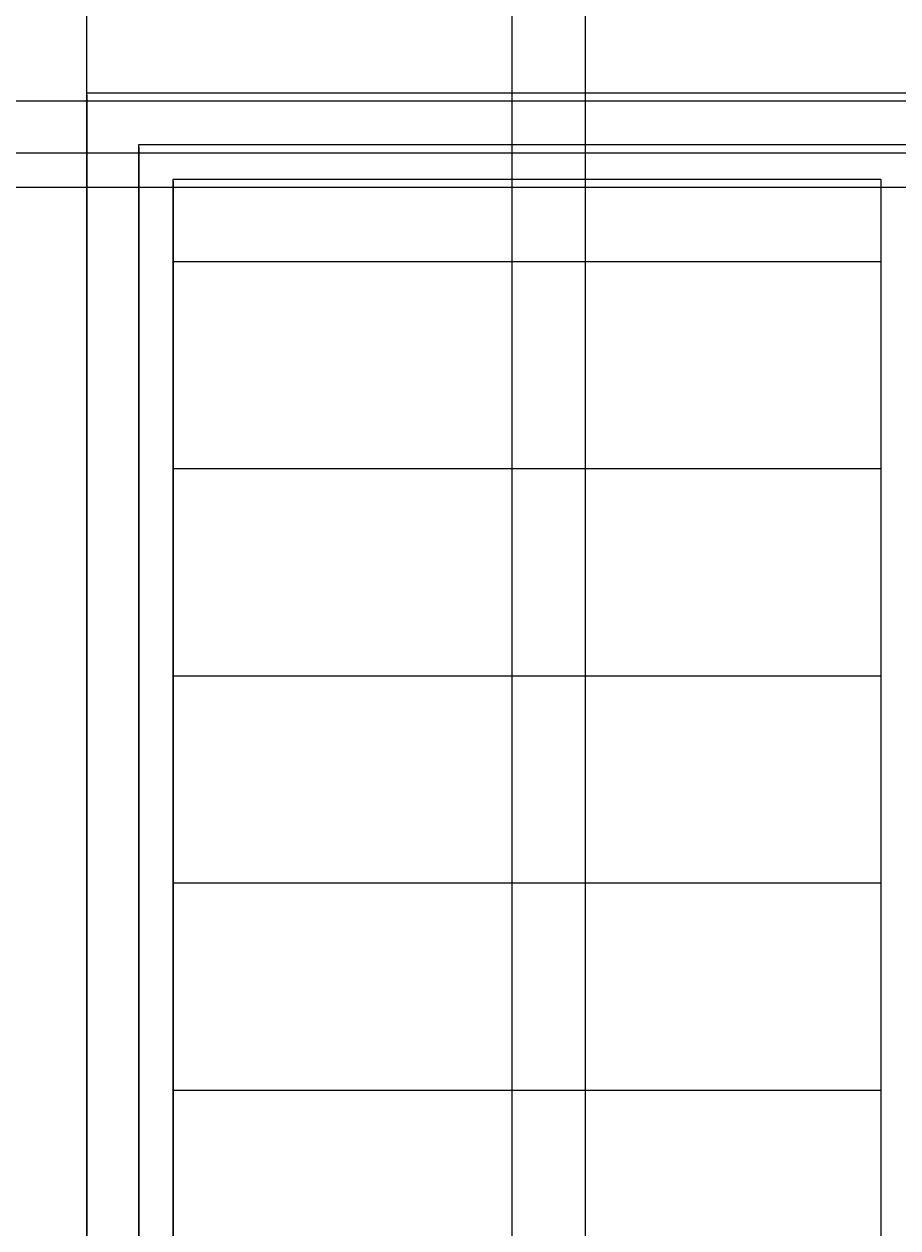
# Model space of a CAD drawing. Units: inches. Extents: x -6 to 289, y -8 to 323.
# Tile 70 of 107: x 186 to 212, y 194 to 229. Entities that reach past the tile are written whole.
import ezdxf

# ---------------------------------------------------------------- set-up
doc = ezdxf.new("R2010")
doc.units = ezdxf.units.IN
doc.header["$MEASUREMENT"] = 0
for name, color, linetype, lineweight in [('A-ANNO-DIMS', 2, 'Continuous', 18), ('A-ELEV-PATT', 8, 'Continuous', 13), ('A-GLAZ', 4, 'Continuous', 25)]:
    doc.layers.add(name, color=color, linetype=linetype, lineweight=lineweight)
doc.styles.get("Standard").update_dxf_attribs({"font": 'arial.ttf'})
doc.dimstyles.get("Standard").update_dxf_attribs({"dimtxt": 0.18, "dimasz": 0.18, "dimexe": 0.18, "dimexo": 0.0625, "dimgap": 0.09, "dimtad": 0, "dimtih": 1, "dimtoh": 1, "dimdec": 4, "dimzin": 0, "dimdsep": 46, "dimtxsty": 'Standard', "dimcen": 0.09, "dimadec": 0, "dimazin": 0, "dimtfac": 1, "dimtdec": 4, "dimtofl": 0, "dimtmove": 0, "dimatfit": 3, "dimfxl": 1, "dimtolj": 1, "dimtzin": 0, "dimarcsym": 0})

# ---------------------------------------------------------------- blocks, each defined once
blk = doc.blocks.new('*D12')
at = {"layer": 'A-ANNO-DIMS', "color": 0, "lineweight": -2, "transparency": 16777216}
for p, q in [((168.883, 226.717), (168.883, 322.969)), ((188.292, 226.951), (188.292, 322.969)), ((169.063, 322.789), (178.22, 322.789)), ((188.112, 322.789), (178.955, 322.789))]:
    blk.add_line(p, q, dxfattribs=at)
at = {"layer": 'A-ANNO-DIMS', "color": 0, "transparency": 16777216}
for points in [[(169.063, 322.819), (169.063, 322.759), (168.883, 322.789)], [(188.112, 322.819), (188.112, 322.759), (188.292, 322.789)]]:
    blk.add_solid(points, dxfattribs=at)
at = {"layer": 'Defpoints', "color": 0, "transparency": 16777216}
for p in [(188.292, 322.789), (168.883, 226.654), (188.292, 226.889)]:
    blk.add_point(p, dxfattribs=at)
at = {"layer": 'A-ANNO-DIMS', "color": 0, "transparency": 16777216, "insert": (178.588, 322.789), "char_height": 0.18, "attachment_point": 5}
blk.add_mtext('\\A1;19.41', dxfattribs=at)
blk = doc.blocks.new('*D13')
at = {"layer": 'A-ANNO-DIMS', "color": 0, "lineweight": -2, "transparency": 16777216}
for p, q in [((188.292, 226.951), (188.292, 322.969)), ((236.292, 226.951), (236.292, 322.969)), ((188.472, 322.789), (212.069, 322.789)), ((236.112, 322.789), (212.515, 322.789))]:
    blk.add_line(p, q, dxfattribs=at)
at = {"layer": 'A-ANNO-DIMS', "color": 0, "transparency": 16777216}
for points in [[(188.472, 322.819), (188.472, 322.759), (188.292, 322.789)], [(236.112, 322.819), (236.112, 322.759), (236.292, 322.789)]]:
    blk.add_solid(points, dxfattribs=at)
at = {"layer": 'Defpoints', "color": 0, "transparency": 16777216}
for p in [(236.292, 322.789), (188.292, 226.889), (236.292, 226.889)]:
    blk.add_point(p, dxfattribs=at)
at = {"layer": 'A-ANNO-DIMS', "color": 0, "transparency": 16777216, "insert": (212.292, 322.789), "char_height": 0.18, "attachment_point": 5}
blk.add_mtext('\\A1;48', dxfattribs=at)
blk = doc.blocks.new('*D25')
at = {"layer": 'A-ANNO-DIMS', "color": 0, "lineweight": -2, "transparency": 16777216}
for p, q in [((126.946, 226.654), (288.653, 226.654)), ((288.473, 226.474), (288.473, 202.836)), ((288.473, 178.834), (288.473, 202.472)), ((126.946, 178.654), (288.653, 178.654))]:
    blk.add_line(p, q, dxfattribs=at)
at = {"layer": 'A-ANNO-DIMS', "color": 0, "transparency": 16777216}
for points in [[(288.443, 226.474), (288.503, 226.474), (288.473, 226.654)], [(288.443, 178.834), (288.503, 178.834), (288.473, 178.654)]]:
    blk.add_solid(points, dxfattribs=at)
at = {"layer": 'Defpoints', "color": 0, "transparency": 16777216}
for p in [(126.883, 226.654), (288.473, 226.654), (126.883, 178.654)]:
    blk.add_point(p, dxfattribs=at)
at = {"layer": 'A-ANNO-DIMS', "color": 0, "transparency": 16777216, "insert": (288.473, 202.654), "char_height": 0.18, "attachment_point": 5}
blk.add_mtext('\\A1;48', dxfattribs=at)
blk = doc.blocks.new('*D26')
at = {"layer": 'A-ANNO-DIMS', "color": 0, "lineweight": -2, "transparency": 16777216}
for p, q in [((247.226, 247.289), (288.653, 247.289)), ((288.473, 247.109), (288.473, 237.153)), ((288.473, 226.834), (288.473, 236.789)), ((126.946, 226.654), (288.653, 226.654))]:
    blk.add_line(p, q, dxfattribs=at)
at = {"layer": 'A-ANNO-DIMS', "color": 0, "transparency": 16777216}
for points in [[(288.443, 247.109), (288.503, 247.109), (288.473, 247.289)], [(288.443, 226.834), (288.503, 226.834), (288.473, 226.654)]]:
    blk.add_solid(points, dxfattribs=at)
at = {"layer": 'Defpoints', "color": 0, "transparency": 16777216}
for p in [(247.164, 247.289), (288.473, 247.289), (126.883, 226.654)]:
    blk.add_point(p, dxfattribs=at)
at = {"layer": 'A-ANNO-DIMS', "color": 0, "transparency": 16777216, "insert": (288.473, 236.971), "char_height": 0.18, "attachment_point": 5}
blk.add_mtext('\\A1;20.635', dxfattribs=at)
blk = doc.blocks.new('*D37')
at = {"layer": 'A-ANNO-DIMS', "color": 0, "lineweight": -2, "transparency": 16777216}
for p, q in [((166.446, 224.154), (288.653, 224.154)), ((288.473, 223.974), (288.473, 202.836)), ((288.473, 181.334), (288.473, 202.472)), ((166.446, 181.154), (288.653, 181.154))]:
    blk.add_line(p, q, dxfattribs=at)
at = {"layer": 'A-ANNO-DIMS', "color": 0, "transparency": 16777216}
for points in [[(288.443, 223.974), (288.503, 223.974), (288.473, 224.154)], [(288.443, 181.334), (288.503, 181.334), (288.473, 181.154)]]:
    blk.add_solid(points, dxfattribs=at)
at = {"layer": 'Defpoints', "color": 0, "transparency": 16777216}
for p in [(166.383, 224.154), (288.473, 224.154), (166.383, 181.154)]:
    blk.add_point(p, dxfattribs=at)
at = {"layer": 'A-ANNO-DIMS', "color": 0, "transparency": 16777216, "insert": (288.473, 202.654), "char_height": 0.18, "attachment_point": 5}
blk.add_mtext('\\A1;43', dxfattribs=at)
blk = doc.blocks.new('*D38')
at = {"layer": 'A-ANNO-DIMS', "color": 0, "lineweight": -2, "transparency": 16777216}
for p, q in [((167.446, 225.154), (288.653, 225.154)), ((288.473, 224.974), (288.473, 224.834)), ((288.473, 224.334), (288.473, 224.474)), ((166.446, 224.154), (288.653, 224.154))]:
    blk.add_line(p, q, dxfattribs=at)
at = {"layer": 'A-ANNO-DIMS', "color": 0, "transparency": 16777216}
for points in [[(288.443, 224.974), (288.503, 224.974), (288.473, 225.154)], [(288.443, 224.334), (288.503, 224.334), (288.473, 224.154)]]:
    blk.add_solid(points, dxfattribs=at)
at = {"layer": 'Defpoints', "color": 0, "transparency": 16777216}
for p in [(167.383, 225.154), (288.473, 225.154), (166.383, 224.154)]:
    blk.add_point(p, dxfattribs=at)
at = {"layer": 'A-ANNO-DIMS', "color": 0, "transparency": 16777216, "insert": (288.473, 224.654), "char_height": 0.18, "attachment_point": 5}
blk.add_mtext('\\A1;1', dxfattribs=at)
blk = doc.blocks.new('*D39')
at = {"layer": 'A-ANNO-DIMS', "color": 0, "lineweight": -2, "transparency": 16777216}
for p, q in [((168.946, 226.654), (288.653, 226.654)), ((288.473, 226.474), (288.473, 226.086)), ((288.473, 225.334), (288.473, 225.722)), ((167.446, 225.154), (288.653, 225.154))]:
    blk.add_line(p, q, dxfattribs=at)
at = {"layer": 'A-ANNO-DIMS', "color": 0, "transparency": 16777216}
for points in [[(288.443, 226.474), (288.503, 226.474), (288.473, 226.654)], [(288.443, 225.334), (288.503, 225.334), (288.473, 225.154)]]:
    blk.add_solid(points, dxfattribs=at)
at = {"layer": 'Defpoints', "color": 0, "transparency": 16777216}
for p in [(168.883, 226.654), (288.473, 226.654), (167.383, 225.154)]:
    blk.add_point(p, dxfattribs=at)
at = {"layer": 'A-ANNO-DIMS', "color": 0, "transparency": 16777216, "insert": (288.473, 225.904), "char_height": 0.18, "attachment_point": 5}
blk.add_mtext('\\A1;1.5', dxfattribs=at)
blk = doc.blocks.new('*D40')
at = {"layer": 'A-ANNO-DIMS', "color": 0, "lineweight": -2, "transparency": 16777216}
for p, q in [((188.292, 226.826), (188.292, -8.391)), ((189.792, 225.326), (189.792, -8.391)), ((188.472, -8.211), (188.796, -8.211)), ((189.612, -8.211), (189.288, -8.211))]:
    blk.add_line(p, q, dxfattribs=at)
at = {"layer": 'A-ANNO-DIMS', "color": 0, "transparency": 16777216}
for points in [[(188.472, -8.181), (188.472, -8.241), (188.292, -8.211)], [(189.612, -8.181), (189.612, -8.241), (189.792, -8.211)]]:
    blk.add_solid(points, dxfattribs=at)
at = {"layer": 'Defpoints', "color": 0, "transparency": 16777216}
for p in [(188.292, 226.889), (189.792, 225.389), (189.792, -8.211)]:
    blk.add_point(p, dxfattribs=at)
at = {"layer": 'A-ANNO-DIMS', "color": 0, "transparency": 16777216, "insert": (189.042, -8.211), "char_height": 0.18, "attachment_point": 5}
blk.add_mtext('\\A1;1.5', dxfattribs=at)
blk = doc.blocks.new('*D41')
at = {"layer": 'A-ANNO-DIMS', "color": 0, "lineweight": -2, "transparency": 16777216}
for p, q in [((189.792, 225.326), (189.792, -8.391)), ((190.792, 224.326), (190.792, -8.391)), ((189.972, -8.211), (190.169, -8.211)), ((190.612, -8.211), (190.415, -8.211))]:
    blk.add_line(p, q, dxfattribs=at)
at = {"layer": 'A-ANNO-DIMS', "color": 0, "transparency": 16777216}
for points in [[(189.972, -8.181), (189.972, -8.241), (189.792, -8.211)], [(190.612, -8.181), (190.612, -8.241), (190.792, -8.211)]]:
    blk.add_solid(points, dxfattribs=at)
at = {"layer": 'Defpoints', "color": 0, "transparency": 16777216}
for p in [(189.792, 225.389), (190.792, 224.389), (190.792, -8.211)]:
    blk.add_point(p, dxfattribs=at)
at = {"layer": 'A-ANNO-DIMS', "color": 0, "transparency": 16777216, "insert": (190.292, -8.211), "char_height": 0.18, "attachment_point": 5}
blk.add_mtext('\\A1;1', dxfattribs=at)
blk = doc.blocks.new('*D42')
at = {"layer": 'A-ANNO-DIMS', "color": 0, "lineweight": -2, "transparency": 16777216}
for p, q in [((190.792, 224.326), (190.792, -8.391)), ((211.292, 224.326), (211.292, -8.391)), ((190.972, -8.211), (200.716, -8.211)), ((211.112, -8.211), (201.368, -8.211))]:
    blk.add_line(p, q, dxfattribs=at)
at = {"layer": 'A-ANNO-DIMS', "color": 0, "transparency": 16777216}
for points in [[(190.972, -8.181), (190.972, -8.241), (190.792, -8.211)], [(211.112, -8.181), (211.112, -8.241), (211.292, -8.211)]]:
    blk.add_solid(points, dxfattribs=at)
at = {"layer": 'Defpoints', "color": 0, "transparency": 16777216}
for p in [(190.792, 224.389), (211.292, 224.389), (211.292, -8.211)]:
    blk.add_point(p, dxfattribs=at)
at = {"layer": 'A-ANNO-DIMS', "color": 0, "transparency": 16777216, "insert": (201.042, -8.211), "char_height": 0.18, "attachment_point": 5}
blk.add_mtext('\\A1;20.5', dxfattribs=at)
blk = doc.blocks.new('*D43')
at = {"layer": 'A-ANNO-DIMS', "color": 0, "lineweight": -2, "transparency": 16777216}
for p, q in [((211.292, 224.326), (211.292, -8.391)), ((212.292, 224.326), (212.292, -8.391)), ((211.472, -8.211), (211.669, -8.211)), ((212.112, -8.211), (211.915, -8.211))]:
    blk.add_line(p, q, dxfattribs=at)
at = {"layer": 'A-ANNO-DIMS', "color": 0, "transparency": 16777216}
for points in [[(211.472, -8.181), (211.472, -8.241), (211.292, -8.211)], [(212.112, -8.181), (212.112, -8.241), (212.292, -8.211)]]:
    blk.add_solid(points, dxfattribs=at)
at = {"layer": 'Defpoints', "color": 0, "transparency": 16777216}
for p in [(211.292, 224.389), (212.292, 224.389), (212.292, -8.211)]:
    blk.add_point(p, dxfattribs=at)
at = {"layer": 'A-ANNO-DIMS', "color": 0, "transparency": 16777216, "insert": (211.792, -8.211), "char_height": 0.18, "attachment_point": 5}
blk.add_mtext('\\A1;1', dxfattribs=at)
blk = doc.blocks.new('*D79')
at = {"layer": 'A-ANNO-DIMS', "color": 0, "lineweight": -2, "transparency": 16777216}
for p, q in [((171.296, 118.033), (171.296, 322.969)), ((188.292, 116.842), (188.292, 322.969)), ((171.476, 322.789), (179.339, 322.789)), ((188.112, 322.789), (180.249, 322.789))]:
    blk.add_line(p, q, dxfattribs=at)
at = {"layer": 'A-ANNO-DIMS', "color": 0, "transparency": 16777216}
for points in [[(171.476, 322.819), (171.476, 322.759), (171.296, 322.789)], [(188.112, 322.819), (188.112, 322.759), (188.292, 322.789)]]:
    blk.add_solid(points, dxfattribs=at)
at = {"layer": 'Defpoints', "color": 0, "transparency": 16777216}
for p in [(188.292, 322.789), (171.296, 117.971), (188.292, 116.779)]:
    blk.add_point(p, dxfattribs=at)
at = {"layer": 'A-ANNO-DIMS', "color": 0, "transparency": 16777216, "insert": (179.794, 322.789), "char_height": 0.18, "attachment_point": 5}
blk.add_mtext('\\A1;16.996', dxfattribs=at)
blk = doc.blocks.new('*D80')
at = {"layer": 'A-ANNO-DIMS', "color": 0, "lineweight": -2, "transparency": 16777216}
for p, q in [((188.292, 116.842), (188.292, 322.969)), ((230.292, 116.842), (230.292, 322.969)), ((188.472, 322.789), (209.07, 322.789)), ((230.112, 322.789), (209.513, 322.789))]:
    blk.add_line(p, q, dxfattribs=at)
at = {"layer": 'A-ANNO-DIMS', "color": 0, "transparency": 16777216}
for points in [[(188.472, 322.819), (188.472, 322.759), (188.292, 322.789)], [(230.112, 322.819), (230.112, 322.759), (230.292, 322.789)]]:
    blk.add_solid(points, dxfattribs=at)
at = {"layer": 'Defpoints', "color": 0, "transparency": 16777216}
for p in [(230.292, 322.789), (188.292, 116.779), (230.292, 116.779)]:
    blk.add_point(p, dxfattribs=at)
at = {"layer": 'A-ANNO-DIMS', "color": 0, "transparency": 16777216, "insert": (209.292, 322.789), "char_height": 0.18, "attachment_point": 5}
blk.add_mtext('\\A1;42', dxfattribs=at)
blk = doc.blocks.new('*D96')
at = {"layer": 'A-ANNO-DIMS', "color": 0, "lineweight": -2, "transparency": 16777216}
for p, q in [((164.004, 159.411), (164.004, 322.969)), ((200.616, 159.411), (200.616, 322.969)), ((164.184, 322.789), (181.934, 322.789)), ((200.436, 322.789), (182.686, 322.789))]:
    blk.add_line(p, q, dxfattribs=at)
at = {"layer": 'A-ANNO-DIMS', "color": 0, "transparency": 16777216}
for points in [[(164.184, 322.819), (164.184, 322.759), (164.004, 322.789)], [(200.436, 322.819), (200.436, 322.759), (200.616, 322.789)]]:
    blk.add_solid(points, dxfattribs=at)
at = {"layer": 'Defpoints', "color": 0, "transparency": 16777216}
for p in [(200.616, 322.789), (164.004, 159.348), (200.616, 159.348)]:
    blk.add_point(p, dxfattribs=at)
at = {"layer": 'A-ANNO-DIMS', "color": 0, "transparency": 16777216, "insert": (182.31, 322.789), "char_height": 0.18, "attachment_point": 5}
blk.add_mtext('\\A1;36.61', dxfattribs=at)
blk = doc.blocks.new('*D97')
at = {"layer": 'A-ANNO-DIMS', "color": 0, "lineweight": -2, "transparency": 16777216}
for p, q in [((200.616, 159.411), (200.616, 322.969)), ((202.741, 159.411), (202.741, 322.969)), ((200.796, 322.789), (201.283, 322.789)), ((202.561, 322.789), (202.075, 322.789))]:
    blk.add_line(p, q, dxfattribs=at)
at = {"layer": 'A-ANNO-DIMS', "color": 0, "transparency": 16777216}
for points in [[(200.796, 322.819), (200.796, 322.759), (200.616, 322.789)], [(202.561, 322.819), (202.561, 322.759), (202.741, 322.789)]]:
    blk.add_solid(points, dxfattribs=at)
at = {"layer": 'Defpoints', "color": 0, "transparency": 16777216}
for p in [(202.741, 322.789), (200.616, 159.348), (202.741, 159.348)]:
    blk.add_point(p, dxfattribs=at)
at = {"layer": 'A-ANNO-DIMS', "color": 0, "transparency": 16777216, "insert": (201.679, 322.789), "char_height": 0.18, "attachment_point": 5}
blk.add_mtext('\\A1;2.125', dxfattribs=at)
blk = doc.blocks.new('*D98')
at = {"layer": 'A-ANNO-DIMS', "color": 0, "lineweight": -2, "transparency": 16777216}
for p, q in [((202.741, 159.411), (202.741, 322.969)), ((244.164, 159.411), (244.164, 322.969)), ((202.921, 322.789), (223.056, 322.789)), ((243.984, 322.789), (223.849, 322.789))]:
    blk.add_line(p, q, dxfattribs=at)
at = {"layer": 'A-ANNO-DIMS', "color": 0, "transparency": 16777216}
for points in [[(202.921, 322.819), (202.921, 322.759), (202.741, 322.789)], [(243.984, 322.819), (243.984, 322.759), (244.164, 322.789)]]:
    blk.add_solid(points, dxfattribs=at)
at = {"layer": 'Defpoints', "color": 0, "transparency": 16777216}
for p in [(244.164, 322.789), (202.741, 159.348), (244.164, 159.348)]:
    blk.add_point(p, dxfattribs=at)
at = {"layer": 'A-ANNO-DIMS', "color": 0, "transparency": 16777216, "insert": (223.452, 322.789), "char_height": 0.18, "attachment_point": 5}
blk.add_mtext('\\A1;41.42', dxfattribs=at)

msp = doc.modelspace()

# ---------------------------------------------------------------- hatches: boundary and pattern name
at = {"layer": 'A-ELEV-PATT'}
h = msp.add_hatch(dxfattribs=at)
h.set_pattern_fill('_USER', color=256, scale=6, pattern_type=0)
h.set_pattern_definition([(0, (0, 0), (0, 6), [])])
h.paths.add_polyline_path([(184.1244, 48.0851), (124.008, 48.0851), (124.008, 10.2888), (184.1244, 10.2888)])
h.paths.add_polyline_path([(244.2408, 48.0851), (186.3604, 48.0851), (186.3604, 10.2888), (244.2408, 10.2888)])
h.paths.add_polyline_path([(208.2918, 114.2795), (190.7918, 114.2795), (190.7918, 71.2795), (208.2918, 71.2795)])
h.paths.add_polyline_path([(227.7918, 114.2795), (209.2918, 114.2795), (209.2918, 71.2795), (227.7918, 71.2795)])
h.paths.add_polyline_path([(211.2918, 224.3887), (190.7918, 224.3887), (190.7918, 162.3484), (211.2918, 162.3484)])
h.paths.add_polyline_path([(233.7918, 224.3887), (212.2918, 224.3887), (212.2918, 162.3484), (233.7918, 162.3484)])
h.paths.add_polyline_path([(166.3835, 224.154), (147.8835, 224.154), (147.8835, 181.154), (166.3835, 181.154)])
h.paths.add_polyline_path([(146.8835, 224.154), (129.3835, 224.154), (129.3835, 181.154), (146.8835, 181.154)])

# ---------------------------------------------------------------- linework, layer by layer
at = {"layer": 'A-GLAZ'}
for p, q in [((189.7918, 225.3887), (212.2918, 225.3887)), ((189.7918, 162.3484), (189.7918, 225.3887))]:
    msp.add_line(p, q, dxfattribs=at)
for points in [[(188.2918, 162.3484), (188.2918, 226.8887), (236.2918, 226.8887), (236.2918, 162.3484)], [(190.7918, 162.3484), (190.7918, 224.3887), (211.2918, 224.3887)], [(211.2918, 224.3887), (211.2918, 162.3484)]]:
    msp.add_lwpolyline(points, dxfattribs=at)

# ---------------------------------------------------------------- dimensions: what is measured, and where the dimension line sits
at = {"layer": 'A-ANNO-DIMS'}
for base, p1, p2, override, picture, middle in [((200.6162, 322.7888), (164.0039, 159.3484), (200.6162, 159.3484), {"dimdec": 2, "dimlfac": 1, "dimrnd": 0, "dimzin": 0, "dimdsep": 46, "dimlunit": 2}, '*D96', (182.3101, 322.7888)), ((188.2918, 322.7888), (168.8835, 226.654), (188.2918, 226.8887), {"dimdec": 2, "dimlfac": 1, "dimrnd": 0, "dimzin": 0, "dimdsep": 46, "dimlunit": 2}, '*D12', (178.5876, 322.7888)), ((188.2918, 322.7888), (171.296, 117.9706), (188.2918, 116.7795), {"dimdec": 3, "dimlfac": 1, "dimrnd": 0, "dimzin": 0, "dimdsep": 46, "dimlunit": 2}, '*D79', (179.7939, 322.7888)), ((236.2918, 322.7888), (188.2918, 226.8887), (236.2918, 226.8887), {"dimdec": 0, "dimlfac": 1, "dimrnd": 0, "dimzin": 0, "dimdsep": 46, "dimlunit": 2}, '*D13', (212.2918, 322.7888)), ((230.2918, 322.7888), (188.2918, 116.7795), (230.2918, 116.7795), {"dimdec": 0, "dimlfac": 1, "dimrnd": 0, "dimzin": 0, "dimdsep": 46, "dimlunit": 2}, '*D80', (209.2918, 322.7888)), ((202.741, 322.7888), (200.6162, 159.3484), (202.741, 159.3484), {"dimdec": 3, "dimlfac": 1, "dimrnd": 0, "dimzin": 0, "dimdsep": 46, "dimlunit": 2}, '*D97', (201.6786, 322.7888)), ((244.1638, 322.7888), (202.741, 159.3484), (244.1638, 159.3484), {"dimdec": 2, "dimlfac": 1, "dimrnd": 0, "dimzin": 0, "dimdsep": 46, "dimlunit": 2}, '*D98', (223.4524, 322.7888)), ((189.7918, -8.2112), (188.2918, 226.8887), (189.7918, 225.3887), {"dimdec": 1, "dimlfac": 1, "dimrnd": 0, "dimzin": 0, "dimdsep": 46, "dimlunit": 2}, '*D40', (189.0418, -8.2112)), ((190.7918, -8.2112), (189.7918, 225.3887), (190.7918, 224.3887), {"dimdec": 0, "dimlfac": 1, "dimrnd": 0, "dimzin": 0, "dimdsep": 46, "dimlunit": 2}, '*D41', (190.2918, -8.2112)), ((211.2918, -8.2112), (190.7918, 224.3887), (211.2918, 224.3887), {"dimdec": 1, "dimlfac": 1, "dimrnd": 0, "dimzin": 0, "dimdsep": 46, "dimlunit": 2}, '*D42', (201.0418, -8.2112)), ((212.2918, -8.2112), (211.2918, 224.3887), (212.2918, 224.3887), {"dimdec": 0, "dimlfac": 1, "dimrnd": 0, "dimzin": 0, "dimdsep": 46, "dimlunit": 2}, '*D43', (211.7918, -8.2112))]:
    dim = msp.add_linear_dim(base=base, p1=p1, p2=p2, dimstyle='Standard', override=override, dxfattribs=at)
    dim.commit()
    dim.dimension.update_dxf_attribs({"geometry": picture, "text_midpoint": middle})
for base, p1, p2, override, picture, middle in [((288.4733, 247.2888), (126.8835, 226.654), (247.1638, 247.2888), {"dimdec": 3, "dimlfac": 1, "dimrnd": 0, "dimzin": 0, "dimdsep": 46, "dimlunit": 2}, '*D26', (288.4733, 236.9714)), ((288.4733, 226.654), (126.8835, 178.654), (126.8835, 226.654), {"dimdec": 0, "dimlfac": 1, "dimrnd": 0, "dimzin": 0, "dimdsep": 46, "dimlunit": 2}, '*D25', (288.4733, 202.654)), ((288.4733, 226.654), (167.3835, 225.154), (168.8835, 226.654), {"dimdec": 1, "dimlfac": 1, "dimrnd": 0, "dimzin": 0, "dimdsep": 46, "dimlunit": 2}, '*D39', (288.4733, 225.904)), ((288.4733, 225.154), (166.3835, 224.154), (167.3835, 225.154), {"dimdec": 0, "dimlfac": 1, "dimrnd": 0, "dimzin": 0, "dimdsep": 46, "dimlunit": 2}, '*D38', (288.4733, 224.654)), ((288.4733, 224.154), (166.3835, 181.154), (166.3835, 224.154), {"dimdec": 0, "dimlfac": 1, "dimrnd": 0, "dimzin": 0, "dimdsep": 46, "dimlunit": 2}, '*D37', (288.4733, 202.654))]:
    dim = msp.add_linear_dim(base=base, p1=p1, p2=p2, angle=90, dimstyle='Standard', override=override, dxfattribs=at)
    dim.commit()
    dim.dimension.update_dxf_attribs({"geometry": picture, "text_midpoint": middle})

doc.saveas('drawing.dxf')
